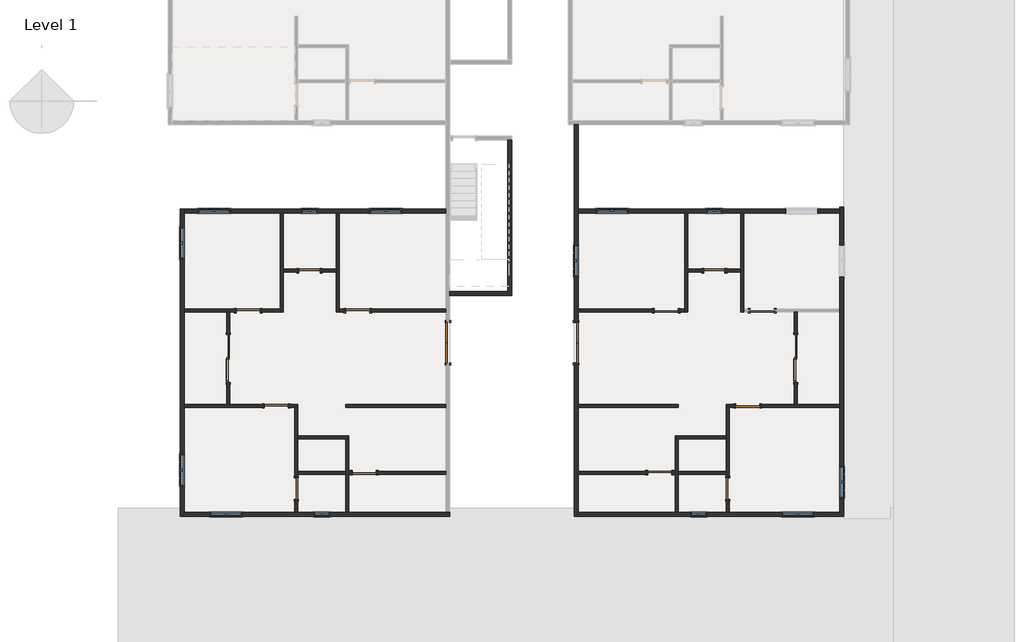
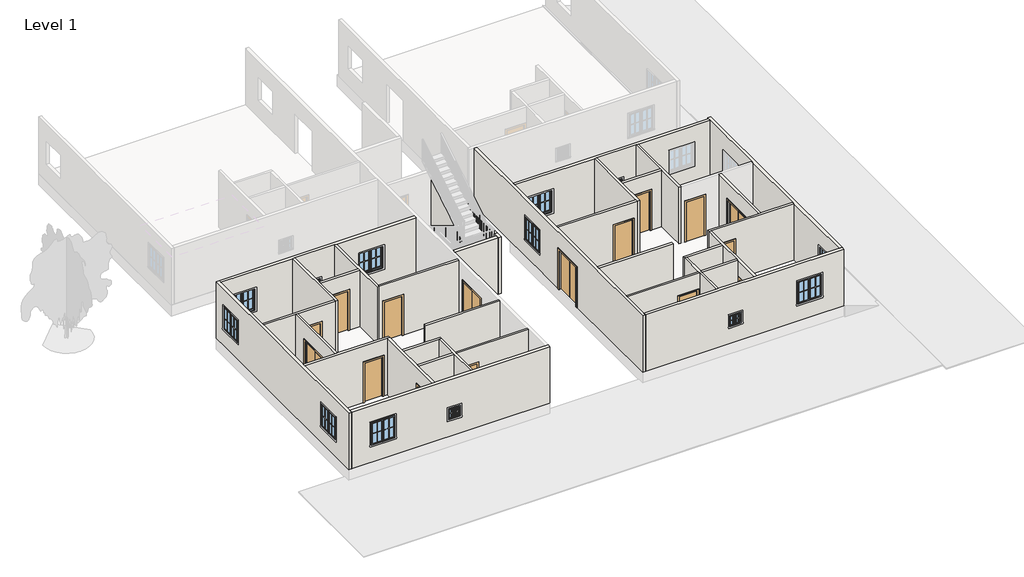
# One storey, part 1 of 7: 32 walls, 16 doors, 13 windows.
"""IFC4 building model written with IfcOpenShell, lengths in millimetres."""

from ifc_helpers import new_model, si_unit, frame, origin, origin_with_axes, place, context, project, spatial, polyline, outline, extrude, faceted_brep, transform, mapped, element, save
from components import door_a09c2f77, door_166d4031, door_d141acb4, door_e5f9f3c4, window_0c121b81, window_191d0cfb

model = new_model("IFC4")

# Units and contexts
model_context = context("Model", 3, world=origin())
ifc_project = project(units=[si_unit("LENGTHUNIT", "METRE", prefix="MILLI")], contexts=[model_context])

# Site, building, storey
site = spatial("IfcSite", under=ifc_project)
building = spatial("IfcBuilding", under=site)
storey = spatial("IfcBuildingStorey", under=building, Name="Level 1", Elevation=0.0)

# Doors
placement = place(None, origin())
door_shape = door_a09c2f77(model_context)
element("IfcDoor", 1, ObjectType="Door-Double-Flush_Panel : 60\" x 84\"", at=placement, inside=storey, context=model_context, shape_type="MappedRepresentation", body=[
    mapped(door_shape, transform((-3579.3844485, -6148.3564015, 0.0), x_axis=(0.0, 1.0, 0.0), y_axis=(-1.0, 0.0, 0.0), z_axis=(0.0, 0.0, 1.0))),
])
element("IfcDoor", 2, ObjectType="Door-Double-Flush_Panel : 60\" x 84\"", at=placement, inside=storey, context=model_context, shape_type="MappedRepresentation", body=[
    mapped(door_shape, transform((1297.4155515, -6148.3564015, 0.0), x_axis=(0.0, -1.0, 0.0), y_axis=(1.0, 0.0, 0.0), z_axis=(0.0, 0.0, 1.0))),
])
door_2_shape = door_166d4031(model_context)
element("IfcDoor", 3, ObjectType="Door-Double-Sliding : 72\" x 84\"", at=placement, inside=storey, context=model_context, shape_type="MappedRepresentation", body=[
    mapped(door_2_shape, transform((-11796.2844485, -6738.9064015, 0.0), x_axis=(0.0, 1.0, 0.0), y_axis=(-1.0, 0.0, 0.0), z_axis=(0.0, 0.0, 1.0))),
])
element("IfcDoor", 4, ObjectType="Door-Double-Sliding : 72\" x 84\"", at=placement, inside=storey, context=model_context, shape_type="MappedRepresentation", body=[
    mapped(door_2_shape, transform((9768.3155515, -6738.9064015, 0.0), x_axis=(0.0, 1.0, 0.0), y_axis=(-1.0, 0.0, 0.0), z_axis=(0.0, 0.0, 1.0))),
])
door_3_shape = door_d141acb4(model_context)
element("IfcDoor", 5, ObjectType="Single-Flush : 32\" x 84\"", at=placement, inside=storey, context=model_context, shape_type="MappedRepresentation", body=[
    mapped(door_3_shape, transform((-8829.5474256, -3405.1564015, 0.0), x_axis=(1.0, 0.0, 0.0), y_axis=(0.0, 1.0, 0.0), z_axis=(0.0, 0.0, 1.0))),
])
element("IfcDoor", 6, ObjectType="Single-Flush : 32\" x 84\"", at=placement, inside=storey, context=model_context, shape_type="MappedRepresentation", body=[
    mapped(door_3_shape, transform((-9338.8344485, -11698.2564015, 0.0), x_axis=(0.0, -1.0, 0.0), y_axis=(1.0, 0.0, 0.0), z_axis=(0.0, 0.0, 1.0))),
])
element("IfcDoor", 7, ObjectType="Single-Flush : 32\" x 84\"", at=placement, inside=storey, context=model_context, shape_type="MappedRepresentation", body=[
    mapped(door_3_shape, transform((7056.8655515, -11698.2564015, 0.0), x_axis=(0.0, 1.0, 0.0), y_axis=(-1.0, 0.0, 0.0), z_axis=(0.0, 0.0, 1.0))),
])
element("IfcDoor", 8, ObjectType="Single-Flush : 32\" x 84\"", at=placement, inside=storey, context=model_context, shape_type="MappedRepresentation", body=[
    mapped(door_3_shape, transform((6547.5785285, -3405.1564015, 0.0), x_axis=(1.0, 0.0, 0.0), y_axis=(0.0, 1.0, 0.0), z_axis=(0.0, 0.0, 1.0))),
])
door_4_shape = door_e5f9f3c4(model_context)
element("IfcDoor", 9, ObjectType="Single-Flush : 36\" x 84\"", at=placement, inside=storey, context=model_context, shape_type="MappedRepresentation", body=[
    mapped(door_4_shape, transform((-11161.2844485, -4929.1564015, 0.0), x_axis=(1.0, 0.0, 0.0), y_axis=(0.0, 1.0, 0.0), z_axis=(0.0, 0.0, 1.0))),
])
element("IfcDoor", 10, ObjectType="Single-Flush : 36\" x 84\"", at=placement, inside=storey, context=model_context, shape_type="MappedRepresentation", body=[
    mapped(door_4_shape, transform((-7007.0974256, -4929.1564015, 0.0), x_axis=(1.0, 0.0, 0.0), y_axis=(0.0, 1.0, 0.0), z_axis=(0.0, 0.0, 1.0))),
])
element("IfcDoor", 11, ObjectType="Single-Flush : 36\" x 84\"", at=placement, inside=storey, context=model_context, shape_type="MappedRepresentation", body=[
    mapped(door_4_shape, transform((-10100.8344485, -8548.6564015, 0.0), x_axis=(1.0, 0.0, 0.0), y_axis=(0.0, 1.0, 0.0), z_axis=(0.0, 0.0, 1.0))),
])
element("IfcDoor", 12, ObjectType="Single-Flush : 36\" x 84\"", at=placement, inside=storey, context=model_context, shape_type="MappedRepresentation", body=[
    mapped(door_4_shape, transform((-6748.0344485, -11088.6564015, 0.0), x_axis=(-1.0, 0.0, 0.0), y_axis=(0.0, -1.0, 0.0), z_axis=(0.0, 0.0, 1.0))),
])
element("IfcDoor", 13, ObjectType="Single-Flush : 36\" x 84\"", at=placement, inside=storey, context=model_context, shape_type="MappedRepresentation", body=[
    mapped(door_4_shape, transform((7818.8655515, -8548.6564015, 0.0), x_axis=(-1.0, 0.0, 0.0), y_axis=(0.0, -1.0, 0.0), z_axis=(0.0, 0.0, 1.0))),
])
element("IfcDoor", 14, ObjectType="Single-Flush : 36\" x 84\"", at=placement, inside=storey, context=model_context, shape_type="MappedRepresentation", body=[
    mapped(door_4_shape, transform((4466.0655515, -11088.6564015, 0.0), x_axis=(1.0, 0.0, 0.0), y_axis=(0.0, 1.0, 0.0), z_axis=(0.0, 0.0, 1.0))),
])
element("IfcDoor", 15, ObjectType="Single-Flush : 36\" x 84\"", at=placement, inside=storey, context=model_context, shape_type="MappedRepresentation", body=[
    mapped(door_4_shape, transform((4725.1285285, -4929.1564015, 0.0), x_axis=(-1.0, 0.0, 0.0), y_axis=(0.0, -1.0, 0.0), z_axis=(0.0, 0.0, 1.0))),
])
element("IfcDoor", 16, ObjectType="Single-Flush : 36\" x 84\"", at=placement, inside=storey, context=model_context, shape_type="MappedRepresentation", body=[
    mapped(door_4_shape, transform((8370.0285285, -4929.1564015, 0.0), x_axis=(-1.0, 0.0, 0.0), y_axis=(0.0, -1.0, 0.0), z_axis=(0.0, 0.0, 1.0))),
])

# Walls
element("IfcWall", 17, ObjectType="4.5\"", at=placement, inside=storey, context=model_context, shape_type="Brep", body=[
    faceted_brep([(-9947.1474256, -1214.4064015, 0.0), (-9947.1474256, -4872.0064015, 0.0), (-9947.1474256, -4986.3064015, 0.0), (-9947.1474256, -4986.3064015, 3048.0), (-9947.1474256, -4872.0064015, 3048.0), (-9947.1474256, -1214.4064015, 3048.0), (-9832.8474256, -1214.4064015, 0.0), (-9832.8474256, -1214.4064015, 3048.0), (-9832.8474256, -3348.0064015, 3048.0), (-9832.8474256, -3462.3064015, 3048.0), (-9832.8474256, -4986.3064015, 3048.0), (-9832.8474256, -4986.3064015, 0.0), (-9832.8474256, -3462.3064015, 0.0), (-9832.8474256, -3348.0064015, 0.0)], [[[0, 1, 2, 3, 4, 5]], [[6, 7, 8, 9, 10, 11, 12, 13]], [[2, 1, 0, 6, 13, 12, 11]], [[0, 5, 7, 6]], [[3, 2, 11, 10]], [[5, 4, 3, 10, 9, 8, 7]]]),
])
element("IfcWall", 18, ObjectType="4.5\"", at=placement, inside=storey, context=model_context, shape_type="Brep", body=[
    faceted_brep([(-9947.1474256, -4872.0064015, 0.0), (-10704.0844485, -4872.0064015, 0.0), (-10704.0844485, -4872.0064015, 2133.6), (-11618.4844485, -4872.0064015, 2133.6), (-11618.4844485, -4872.0064015, 0.0), (-13604.1663899, -4872.0064015, 0.0), (-13604.1663899, -4872.0064015, 3048.0), (-9947.1474256, -4872.0064015, 3048.0), (-10704.0844485, -4986.3064015, 2133.6), (-10704.0844485, -4986.3064015, 0.0), (-9947.1474256, -4986.3064015, 0.0), (-9947.1474256, -4986.3064015, 3048.0), (-11866.1344485, -4986.3064015, 3048.0), (-11980.4344485, -4986.3064015, 3048.0), (-13604.1663899, -4986.3064015, 3048.0), (-13604.1663899, -4986.3064015, 0.0), (-11980.4344485, -4986.3064015, 0.0), (-11866.1344485, -4986.3064015, 0.0), (-11618.4844485, -4986.3064015, 0.0), (-11618.4844485, -4986.3064015, 2133.6)], [[[0, 1, 2, 3, 4, 5, 6, 7]], [[8, 9, 10, 11, 12, 13, 14, 15, 16, 17, 18, 19]], [[10, 9, 1, 0]], [[18, 17, 16, 15, 5, 4]], [[0, 7, 11, 10]], [[6, 5, 15, 14]], [[2, 1, 9, 8]], [[3, 2, 8, 19]], [[4, 3, 19, 18]], [[7, 6, 14, 13, 12, 11]]]),
])
element("IfcWall", 19, ObjectType="4.5\"", at=placement, inside=storey, context=model_context, shape_type="SweptSolid", body=[
    extrude(outline(polyline([(-4986.3064015, 0.0), (-5824.5064015, 0.0), (-5824.5064015, 2133.6), (-7653.3064015, 2133.6), (-7653.3064015, 0.0), (-8491.5064015, 0.0), (-8491.5064015, 3048.0), (-4986.3064015, 3048.0), (-4986.3064015, 0.0)])), frame((-11980.4344485, 0.0, 0.0), z_axis=(1.0, 0.0, 0.0), x_axis=(0.0, 1.0, 0.0)), (0.0, 0.0, 1.0), 114.3),
])
element("IfcWall", 20, ObjectType="4.5\"", at=placement, inside=storey, context=model_context, shape_type="SweptSolid", body=[
    extrude(outline(polyline([(2133.6, -8423.1474256), (0.0, -8423.1474256), (0.0, -7826.2474256), (3048.0, -7826.2474256), (3048.0, -9832.8474256), (0.0, -9832.8474256), (0.0, -9235.9474256), (2133.6, -9235.9474256), (2133.6, -8423.1474256)])), frame((0.0, -3462.3064015, 0.0), z_axis=(0.0, 1.0, 0.0), x_axis=(0.0, 0.0, 1.0)), (0.0, 0.0, 1.0), 114.3),
])
element("IfcWall", 21, ObjectType="4.5\"", at=placement, inside=storey, context=model_context, shape_type="Brep", body=[
    faceted_brep([(-7826.2474256, -1214.4064015, 0.0), (-7826.2474256, -3348.0064015, 0.0), (-7826.2474256, -3462.3064015, 0.0), (-7826.2474256, -4986.3064015, 0.0), (-7826.2474256, -4986.3064015, 3048.0), (-7826.2474256, -3462.3064015, 3048.0), (-7826.2474256, -3348.0064015, 3048.0), (-7826.2474256, -1214.4064015, 3048.0), (-7711.9474256, -1214.4064015, 0.0), (-7711.9474256, -1214.4064015, 3048.0), (-7711.9474256, -4872.0064015, 3048.0), (-7711.9474256, -4986.3064015, 3048.0), (-7711.9474256, -4986.3064015, 0.0), (-7711.9474256, -4872.0064015, 0.0)], [[[0, 1, 2, 3, 4, 5, 6, 7]], [[8, 9, 10, 11, 12, 13]], [[3, 2, 1, 0, 8, 13, 12]], [[0, 7, 9, 8]], [[4, 3, 12, 11]], [[7, 6, 5, 4, 11, 10, 9]]]),
])
element("IfcWall", 22, ObjectType="4.5\"", at=placement, inside=storey, context=model_context, shape_type="SweptSolid", body=[
    extrude(outline(polyline([(2133.6, -6549.8974256), (0.0, -6549.8974256), (0.0, -3655.5844485), (3048.0, -3655.5844485), (3048.0, -7711.9474256), (0.0, -7711.9474256), (0.0, -7464.2974256), (2133.6, -7464.2974256), (2133.6, -6549.8974256)])), frame((0.0, -4986.3064015, 0.0), z_axis=(0.0, 1.0, 0.0), x_axis=(0.0, 0.0, 1.0)), (0.0, 0.0, 1.0), 114.3),
])
element("IfcWall", 23, ObjectType="4.5\"", at=placement, inside=storey, context=model_context, shape_type="Brep", body=[
    faceted_brep([(-9643.6344485, -8605.8064015, 2133.6), (-9643.6344485, -8605.8064015, 0.0), (-9395.9844485, -8605.8064015, 0.0), (-9281.6844485, -8605.8064015, 0.0), (-9281.6844485, -8605.8064015, 3048.0), (-9395.9844485, -8605.8064015, 3048.0), (-13604.1663899, -8605.8064015, 3048.0), (-13604.1663899, -8605.8064015, 0.0), (-10558.0344485, -8605.8064015, 0.0), (-10558.0344485, -8605.8064015, 2133.6), (-9281.6844485, -8491.5064015, 0.0), (-9643.6344485, -8491.5064015, 0.0), (-9643.6344485, -8491.5064015, 2133.6), (-10558.0344485, -8491.5064015, 2133.6), (-10558.0344485, -8491.5064015, 0.0), (-11866.1344485, -8491.5064015, 0.0), (-11980.4344485, -8491.5064015, 0.0), (-13604.1663899, -8491.5064015, 0.0), (-13604.1663899, -8491.5064015, 3048.0), (-11980.4344485, -8491.5064015, 3048.0), (-11866.1344485, -8491.5064015, 3048.0), (-9281.6844485, -8491.5064015, 3048.0)], [[[0, 1, 2, 3, 4, 5, 6, 7, 8, 9]], [[10, 11, 12, 13, 14, 15, 16, 17, 18, 19, 20, 21]], [[8, 7, 17, 16, 15, 14]], [[3, 2, 1, 11, 10]], [[7, 6, 18, 17]], [[4, 3, 10, 21]], [[12, 11, 1, 0]], [[13, 12, 0, 9]], [[14, 13, 9, 8]], [[6, 5, 4, 21, 20, 19, 18]]]),
])
element("IfcWall", 24, ObjectType="4.5\"", at=placement, inside=storey, context=model_context, shape_type="Brep", body=[
    faceted_brep([(-9395.9844485, -12104.6564015, 2133.6), (-9395.9844485, -12104.6564015, 0.0), (-9395.9844485, -12593.6064015, 0.0), (-9395.9844485, -12593.6064015, 3048.0), (-9395.9844485, -8605.8064015, 3048.0), (-9395.9844485, -8605.8064015, 0.0), (-9395.9844485, -11291.8564015, 0.0), (-9395.9844485, -11291.8564015, 2133.6), (-9281.6844485, -12593.6064015, 0.0), (-9281.6844485, -12104.6564015, 0.0), (-9281.6844485, -12104.6564015, 2133.6), (-9281.6844485, -11291.8564015, 2133.6), (-9281.6844485, -11291.8564015, 0.0), (-9281.6844485, -11145.8064015, 0.0), (-9281.6844485, -11031.5064015, 0.0), (-9281.6844485, -9812.3064015, 0.0), (-9281.6844485, -9698.0064015, 0.0), (-9281.6844485, -8605.8064015, 0.0), (-9281.6844485, -8605.8064015, 3048.0), (-9281.6844485, -9698.0064015, 3048.0), (-9281.6844485, -9812.3064015, 3048.0), (-9281.6844485, -11031.5064015, 3048.0), (-9281.6844485, -11145.8064015, 3048.0), (-9281.6844485, -12593.6064015, 3048.0)], [[[0, 1, 2, 3, 4, 5, 6, 7]], [[8, 9, 10, 11, 12, 13, 14, 15, 16, 17, 18, 19, 20, 21, 22, 23]], [[6, 5, 17, 16, 15, 14, 13, 12]], [[2, 1, 9, 8]], [[5, 4, 18, 17]], [[3, 2, 8, 23]], [[10, 9, 1, 0]], [[11, 10, 0, 7]], [[12, 11, 7, 6]], [[4, 3, 23, 22, 21, 20, 19, 18]]]),
])
element("IfcWall", 25, ObjectType="4.5\"", at=placement, inside=storey, context=model_context, shape_type="Brep", body=[
    faceted_brep([(-9281.6844485, -9812.3064015, 0.0), (-7452.8844485, -9812.3064015, 0.0), (-7338.5844485, -9812.3064015, 0.0), (-7338.5844485, -9812.3064015, 3048.0), (-7452.8844485, -9812.3064015, 3048.0), (-9281.6844485, -9812.3064015, 3048.0), (-9281.6844485, -9698.0064015, 0.0), (-9281.6844485, -9698.0064015, 3048.0), (-7338.5844485, -9698.0064015, 3048.0), (-7338.5844485, -9698.0064015, 0.0)], [[[0, 1, 2, 3, 4, 5]], [[6, 7, 8, 9]], [[2, 1, 0, 6, 9]], [[0, 5, 7, 6]], [[3, 2, 9, 8]], [[5, 4, 3, 8, 7]]]),
])
element("IfcWall", 26, ObjectType="4.5\"", at=placement, inside=storey, context=model_context, shape_type="Brep", body=[
    faceted_brep([(-7452.8844485, -9812.3064015, 0.0), (-7452.8844485, -11031.5064015, 0.0), (-7452.8844485, -11145.8064015, 0.0), (-7452.8844485, -12593.6064015, 0.0), (-7452.8844485, -12593.6064015, 3048.0), (-7452.8844485, -11145.8064015, 3048.0), (-7452.8844485, -11031.5064015, 3048.0), (-7452.8844485, -9812.3064015, 3048.0), (-7338.5844485, -9812.3064015, 0.0), (-7338.5844485, -9812.3064015, 3048.0), (-7338.5844485, -11031.5064015, 3048.0), (-7338.5844485, -11145.8064015, 3048.0), (-7338.5844485, -12593.6064015, 3048.0), (-7338.5844485, -12593.6064015, 0.0), (-7338.5844485, -11145.8064015, 0.0), (-7338.5844485, -11031.5064015, 0.0)], [[[0, 1, 2, 3, 4, 5, 6, 7]], [[8, 9, 10, 11, 12, 13, 14, 15]], [[3, 2, 1, 0, 8, 15, 14, 13]], [[0, 7, 9, 8]], [[4, 3, 13, 12]], [[7, 6, 5, 4, 12, 11, 10, 9]]]),
])
element("IfcWall", 27, ObjectType="4.5\"", at=placement, inside=storey, context=model_context, shape_type="SweptSolid", body=[
    extrude(outline(polyline([(0.0, -3655.5844485), (3048.0, -3655.5844485), (3048.0, -7338.5844485), (0.0, -7338.5844485), (0.0, -7205.2344485), (2133.6, -7205.2344485), (2133.6, -6290.8344485), (0.0, -6290.8344485), (0.0, -3655.5844485)])), frame((0.0, -11145.8064015, 0.0), z_axis=(0.0, 1.0, 0.0), x_axis=(0.0, 0.0, 1.0)), (0.0, 0.0, 1.0), 114.3),
    extrude(outline(polyline([(-9281.6844485, -11145.8064015), (-9281.6844485, -11031.5064015), (-7452.8844485, -11031.5064015), (-7452.8844485, -11145.8064015), (-9281.6844485, -11145.8064015)])), origin_with_axes(), (0.0, 0.0, 1.0), 3048.0),
])
element("IfcWall", 28, ObjectType="4.5\"", at=placement, inside=storey, context=model_context, shape_type="SweptSolid", body=[
    extrude(outline(polyline([(-3655.5844485, -8605.8064015), (-7452.8844485, -8605.8064015), (-7452.8844485, -8491.5064015), (-3655.5844485, -8491.5064015), (-3655.5844485, -8605.8064015)])), origin_with_axes(), (0.0, 0.0, 1.0), 3048.0),
])
element("IfcWall", 29, ObjectType="4.5\"", at=placement, inside=storey, context=model_context, shape_type="Brep", body=[
    faceted_brep([(5429.9785285, -1214.4064015, 0.0), (5429.9785285, -4872.0064015, 0.0), (5429.9785285, -4986.3064015, 0.0), (5429.9785285, -4986.3064015, 3048.0), (5429.9785285, -4872.0064015, 3048.0), (5429.9785285, -1214.4064015, 3048.0), (5544.2785285, -1214.4064015, 0.0), (5544.2785285, -1214.4064015, 3048.0), (5544.2785285, -3348.0064015, 3048.0), (5544.2785285, -3462.3064015, 3048.0), (5544.2785285, -4986.3064015, 3048.0), (5544.2785285, -4986.3064015, 0.0), (5544.2785285, -3462.3064015, 0.0), (5544.2785285, -3348.0064015, 0.0)], [[[0, 1, 2, 3, 4, 5]], [[6, 7, 8, 9, 10, 11, 12, 13]], [[2, 1, 0, 6, 13, 12, 11]], [[0, 5, 7, 6]], [[3, 2, 11, 10]], [[5, 4, 3, 10, 9, 8, 7]]]),
])
element("IfcWall", 30, ObjectType="4.5\"", at=placement, inside=storey, context=model_context, shape_type="SweptSolid", body=[
    extrude(outline(polyline([(0.0, 1373.6155515), (0.0, 4267.9285285), (2133.6, 4267.9285285), (2133.6, 5182.3285285), (0.0, 5182.3285285), (0.0, 5429.9785285), (3048.0, 5429.9785285), (3048.0, 1373.6155515), (0.0, 1373.6155515)])), frame((0.0, -4986.3064015, 0.0), z_axis=(0.0, 1.0, 0.0), x_axis=(0.0, 0.0, 1.0)), (0.0, 0.0, 1.0), 114.3),
])
element("IfcWall", 31, ObjectType="4.5\"", at=placement, inside=storey, context=model_context, shape_type="Brep", body=[
    faceted_brep([(7550.8785285, -1214.4064015, 0.0), (7550.8785285, -3348.0064015, 0.0), (7550.8785285, -3462.3064015, 0.0), (7550.8785285, -4986.3064015, 0.0), (7550.8785285, -4986.3064015, 3048.0), (7550.8785285, -3462.3064015, 3048.0), (7550.8785285, -3348.0064015, 3048.0), (7550.8785285, -1214.4064015, 3048.0), (7665.1785285, -1214.4064015, 0.0), (7665.1785285, -1214.4064015, 3048.0), (7665.1785285, -4872.0064015, 3048.0), (7665.1785285, -4986.3064015, 3048.0), (7665.1785285, -4986.3064015, 0.0), (7665.1785285, -4872.0064015, 0.0)], [[[0, 1, 2, 3, 4, 5, 6, 7]], [[8, 9, 10, 11, 12, 13]], [[3, 2, 1, 0, 8, 13, 12]], [[0, 7, 9, 8]], [[4, 3, 12, 11]], [[7, 6, 5, 4, 11, 10, 9]]]),
])
element("IfcWall", 32, ObjectType="4.5\"", at=placement, inside=storey, context=model_context, shape_type="SweptSolid", body=[
    extrude(outline(polyline([(2133.6, 6953.9785285), (0.0, 6953.9785285), (0.0, 7550.8785285), (3048.0, 7550.8785285), (3048.0, 5544.2785285), (0.0, 5544.2785285), (0.0, 6141.1785285), (2133.6, 6141.1785285), (2133.6, 6953.9785285)])), frame((0.0, -3462.3064015, 0.0), z_axis=(0.0, 1.0, 0.0), x_axis=(0.0, 0.0, 1.0)), (0.0, 0.0, 1.0), 114.3),
])
element("IfcWall", 33, ObjectType="4.5\"", at=placement, inside=storey, context=model_context, shape_type="SweptSolid", body=[
    extrude(outline(polyline([(-4986.3064015, 0.0), (-5824.5064015, 0.0), (-5824.5064015, 2133.6), (-7653.3064015, 2133.6), (-7653.3064015, 0.0), (-8491.5064015, 0.0), (-8491.5064015, 3048.0), (-4986.3064015, 3048.0), (-4986.3064015, 0.0)])), frame((9584.1655515, 0.0, 0.0), z_axis=(1.0, 0.0, 0.0), x_axis=(0.0, 1.0, 0.0)), (0.0, 0.0, 1.0), 114.3),
])
element("IfcWall", 34, ObjectType="4.5\"", at=placement, inside=storey, context=model_context, shape_type="Brep", body=[
    faceted_brep([(7361.6655515, -8491.5064015, 2133.6), (7361.6655515, -8491.5064015, 0.0), (6999.7155515, -8491.5064015, 0.0), (6999.7155515, -8491.5064015, 3048.0), (9584.1655515, -8491.5064015, 3048.0), (9698.4655515, -8491.5064015, 3048.0), (11322.7785285, -8491.5064015, 3048.0), (11322.7785285, -8491.5064015, 0.0), (9698.4655515, -8491.5064015, 0.0), (9584.1655515, -8491.5064015, 0.0), (8276.0655515, -8491.5064015, 0.0), (8276.0655515, -8491.5064015, 2133.6), (6999.7155515, -8605.8064015, 0.0), (7114.0155515, -8605.8064015, 0.0), (7361.6655515, -8605.8064015, 0.0), (7361.6655515, -8605.8064015, 2133.6), (8276.0655515, -8605.8064015, 2133.6), (8276.0655515, -8605.8064015, 0.0), (11322.7785285, -8605.8064015, 0.0), (11322.7785285, -8605.8064015, 3048.0), (7114.0155515, -8605.8064015, 3048.0), (6999.7155515, -8605.8064015, 3048.0)], [[[0, 1, 2, 3, 4, 5, 6, 7, 8, 9, 10, 11]], [[12, 13, 14, 15, 16, 17, 18, 19, 20, 21]], [[2, 1, 14, 13, 12]], [[10, 9, 8, 7, 18, 17]], [[7, 6, 19, 18]], [[3, 2, 12, 21]], [[15, 14, 1, 0]], [[16, 15, 0, 11]], [[17, 16, 11, 10]], [[6, 5, 4, 3, 21, 20, 19]]]),
])
element("IfcWall", 35, ObjectType="4.5\"", at=placement, inside=storey, context=model_context, shape_type="Brep", body=[
    faceted_brep([(6999.7155515, -8605.8064015, 0.0), (6999.7155515, -9698.0064015, 0.0), (6999.7155515, -9812.3064015, 0.0), (6999.7155515, -11031.5064015, 0.0), (6999.7155515, -11145.8064015, 0.0), (6999.7155515, -11291.8564015, 0.0), (6999.7155515, -11291.8564015, 2133.6), (6999.7155515, -12104.6564015, 2133.6), (6999.7155515, -12104.6564015, 0.0), (6999.7155515, -12593.6064015, 0.0), (6999.7155515, -12593.6064015, 3048.0), (6999.7155515, -11145.8064015, 3048.0), (6999.7155515, -11031.5064015, 3048.0), (6999.7155515, -9812.3064015, 3048.0), (6999.7155515, -9698.0064015, 3048.0), (6999.7155515, -8605.8064015, 3048.0), (7114.0155515, -11291.8564015, 2133.6), (7114.0155515, -11291.8564015, 0.0), (7114.0155515, -8605.8064015, 0.0), (7114.0155515, -8605.8064015, 3048.0), (7114.0155515, -12593.6064015, 3048.0), (7114.0155515, -12593.6064015, 0.0), (7114.0155515, -12104.6564015, 0.0), (7114.0155515, -12104.6564015, 2133.6)], [[[0, 1, 2, 3, 4, 5, 6, 7, 8, 9, 10, 11, 12, 13, 14, 15]], [[16, 17, 18, 19, 20, 21, 22, 23]], [[22, 21, 9, 8]], [[18, 17, 5, 4, 3, 2, 1, 0]], [[0, 15, 19, 18]], [[10, 9, 21, 20]], [[6, 5, 17, 16]], [[7, 6, 16, 23]], [[8, 7, 23, 22]], [[15, 14, 13, 12, 11, 10, 20, 19]]]),
])
element("IfcWall", 36, ObjectType="4.5\"", at=placement, inside=storey, context=model_context, shape_type="Brep", body=[
    faceted_brep([(6999.7155515, -9698.0064015, 0.0), (5056.6155515, -9698.0064015, 0.0), (5056.6155515, -9698.0064015, 3048.0), (6999.7155515, -9698.0064015, 3048.0), (6999.7155515, -9812.3064015, 0.0), (6999.7155515, -9812.3064015, 3048.0), (5170.9155515, -9812.3064015, 3048.0), (5056.6155515, -9812.3064015, 3048.0), (5056.6155515, -9812.3064015, 0.0), (5170.9155515, -9812.3064015, 0.0)], [[[0, 1, 2, 3]], [[4, 5, 6, 7, 8, 9]], [[1, 0, 4, 9, 8]], [[0, 3, 5, 4]], [[2, 1, 8, 7]], [[3, 2, 7, 6, 5]]]),
])
element("IfcWall", 37, ObjectType="4.5\"", at=placement, inside=storey, context=model_context, shape_type="Brep", body=[
    faceted_brep([(5056.6155515, -9812.3064015, 0.0), (5056.6155515, -11031.5064015, 0.0), (5056.6155515, -11145.8064015, 0.0), (5056.6155515, -12593.6064015, 0.0), (5056.6155515, -12593.6064015, 3048.0), (5056.6155515, -11145.8064015, 3048.0), (5056.6155515, -11031.5064015, 3048.0), (5056.6155515, -9812.3064015, 3048.0), (5170.9155515, -9812.3064015, 0.0), (5170.9155515, -9812.3064015, 3048.0), (5170.9155515, -11031.5064015, 3048.0), (5170.9155515, -11145.8064015, 3048.0), (5170.9155515, -12593.6064015, 3048.0), (5170.9155515, -12593.6064015, 0.0), (5170.9155515, -11145.8064015, 0.0), (5170.9155515, -11031.5064015, 0.0)], [[[0, 1, 2, 3, 4, 5, 6, 7]], [[8, 9, 10, 11, 12, 13, 14, 15]], [[3, 2, 1, 0, 8, 15, 14, 13]], [[0, 7, 9, 8]], [[4, 3, 13, 12]], [[7, 6, 5, 4, 12, 11, 10, 9]]]),
])
element("IfcWall", 38, ObjectType="4.5\"", at=placement, inside=storey, context=model_context, shape_type="SweptSolid", body=[
    extrude(outline(polyline([(3048.0, 1373.6155515), (0.0, 1373.6155515), (0.0, 4008.8655515), (2133.6, 4008.8655515), (2133.6, 4923.2655515), (0.0, 4923.2655515), (0.0, 5056.6155515), (3048.0, 5056.6155515), (3048.0, 1373.6155515)])), frame((0.0, -11145.8064015, 0.0), z_axis=(0.0, 1.0, 0.0), x_axis=(0.0, 0.0, 1.0)), (0.0, 0.0, 1.0), 114.3),
    extrude(outline(polyline([(6999.7155515, -11031.5064015), (6999.7155515, -11145.8064015), (5170.9155515, -11145.8064015), (5170.9155515, -11031.5064015), (6999.7155515, -11031.5064015)])), origin_with_axes(), (0.0, 0.0, 1.0), 3048.0),
])
element("IfcWall", 39, ObjectType="4.5\"", at=placement, inside=storey, context=model_context, shape_type="SweptSolid", body=[
    extrude(outline(polyline([(5170.9155515, -8605.8064015), (1373.6155515, -8605.8064015), (1373.6155515, -8491.5064015), (5170.9155515, -8491.5064015), (5170.9155515, -8605.8064015)])), origin_with_axes(), (0.0, 0.0, 1.0), 3048.0),
])
element("IfcWall", 40, ObjectType="6\"", at=placement, inside=storey, context=model_context, shape_type="Brep", body=[
    faceted_brep([(-13756.5663899, -1055.4730729, 0.0), (-13756.5663899, -12746.0064015, 0.0), (-13756.5663899, -12746.0064015, 3048.0), (-13756.5663899, -1055.4730729, 3048.0), (-13756.5663899, -1747.8317701, 2133.6), (-13756.5663899, -2967.0317701, 2133.6), (-13756.5663899, -2967.0317701, 914.4), (-13756.5663899, -1747.8317701, 914.4), (-13756.5663899, -10383.8317701, 2133.6), (-13756.5663899, -11603.0317701, 2133.6), (-13756.5663899, -11603.0317701, 914.4), (-13756.5663899, -10383.8317701, 914.4), (-13604.1663899, -1055.4730729, 0.0), (-13604.1663899, -1055.4730729, 3048.0), (-13604.1663899, -1062.0064015, 3048.0), (-13604.1663899, -1214.4064015, 3048.0), (-13604.1663899, -4872.0064015, 3048.0), (-13604.1663899, -4986.3064015, 3048.0), (-13604.1663899, -8491.5064015, 3048.0), (-13604.1663899, -8605.8064015, 3048.0), (-13604.1663899, -12593.6064015, 3048.0), (-13604.1663899, -12746.0064015, 3048.0), (-13604.1663899, -12746.0064015, 0.0), (-13604.1663899, -12593.6064015, 0.0), (-13604.1663899, -8605.8064015, 0.0), (-13604.1663899, -8491.5064015, 0.0), (-13604.1663899, -4986.3064015, 0.0), (-13604.1663899, -4872.0064015, 0.0), (-13604.1663899, -1214.4064015, 0.0), (-13604.1663899, -1062.0064015, 0.0), (-13604.1663899, -1747.8317701, 2133.6), (-13604.1663899, -1747.8317701, 914.4), (-13604.1663899, -2967.0317701, 914.4), (-13604.1663899, -2967.0317701, 2133.6), (-13604.1663899, -10383.8317701, 2133.6), (-13604.1663899, -10383.8317701, 914.4), (-13604.1663899, -11603.0317701, 914.4), (-13604.1663899, -11603.0317701, 2133.6)], [[[0, 1, 2, 3], [4, 5, 6, 7], [8, 9, 10, 11]], [[12, 13, 14, 15, 16, 17, 18, 19, 20, 21, 22, 23, 24, 25, 26, 27, 28, 29], [30, 31, 32, 33], [34, 35, 36, 37]], [[1, 0, 12, 29, 28, 27, 26, 25, 24, 23, 22]], [[0, 3, 13, 12]], [[2, 1, 22, 21]], [[31, 30, 4, 7]], [[32, 31, 7, 6]], [[33, 32, 6, 5]], [[30, 33, 5, 4]], [[35, 34, 8, 11]], [[36, 35, 11, 10]], [[37, 36, 10, 9]], [[34, 37, 9, 8]], [[3, 2, 21, 20, 19, 18, 17, 16, 15, 14, 13]]]),
])
element("IfcWall", 41, ObjectType="6\"", at=placement, inside=storey, context=model_context, shape_type="Brep", body=[
    faceted_brep([(-13604.1663899, -12746.0064015, 0.0), (-3503.1844485, -12746.0064015, 0.0), (-3503.1844485, -12746.0064015, 3048.0), (-13604.1663899, -12746.0064015, 3048.0), (-12614.1474256, -12746.0064015, 2133.6), (-11394.9474256, -12746.0064015, 2133.6), (-11394.9474256, -12746.0064015, 914.4), (-12614.1474256, -12746.0064015, 914.4), (-8672.0844485, -12746.0064015, 1524.0), (-8062.4844485, -12746.0064015, 1524.0), (-8062.4844485, -12746.0064015, 914.4), (-8672.0844485, -12746.0064015, 914.4), (-13604.1663899, -12593.6064015, 0.0), (-13604.1663899, -12593.6064015, 3048.0), (-9395.9844485, -12593.6064015, 3048.0), (-9281.6844485, -12593.6064015, 3048.0), (-7452.8844485, -12593.6064015, 3048.0), (-7338.5844485, -12593.6064015, 3048.0), (-3655.5844485, -12593.6064015, 3048.0), (-3503.1844485, -12593.6064015, 3048.0), (-3503.1844485, -12593.6064015, 0.0), (-3655.5844485, -12593.6064015, 0.0), (-7338.5844485, -12593.6064015, 0.0), (-7452.8844485, -12593.6064015, 0.0), (-9281.6844485, -12593.6064015, 0.0), (-9395.9844485, -12593.6064015, 0.0), (-12614.1474256, -12593.6064015, 2133.6), (-12614.1474256, -12593.6064015, 914.4), (-11394.9474256, -12593.6064015, 914.4), (-11394.9474256, -12593.6064015, 2133.6), (-8672.0844485, -12593.6064015, 1524.0), (-8672.0844485, -12593.6064015, 914.4), (-8062.4844485, -12593.6064015, 914.4), (-8062.4844485, -12593.6064015, 1524.0)], [[[0, 1, 2, 3], [4, 5, 6, 7], [8, 9, 10, 11]], [[12, 13, 14, 15, 16, 17, 18, 19, 20, 21, 22, 23, 24, 25], [26, 27, 28, 29], [30, 31, 32, 33]], [[1, 0, 12, 25, 24, 23, 22, 21, 20]], [[0, 3, 13, 12]], [[2, 1, 20, 19]], [[27, 26, 4, 7]], [[28, 27, 7, 6]], [[29, 28, 6, 5]], [[26, 29, 5, 4]], [[31, 30, 8, 11]], [[32, 31, 11, 10]], [[33, 32, 10, 9]], [[30, 33, 9, 8]], [[3, 2, 19, 18, 17, 16, 15, 14, 13]]]),
])
element("IfcWall", 42, ObjectType="6\"", at=placement, inside=storey, context=model_context, shape_type="Brep", body=[
    faceted_brep([(-13604.1663899, -1214.4064015, 0.0), (-9947.1474256, -1214.4064015, 0.0), (-9832.8474256, -1214.4064015, 0.0), (-7826.2474256, -1214.4064015, 0.0), (-7711.9474256, -1214.4064015, 0.0), (-3655.5844485, -1214.4064015, 0.0), (-3655.5844485, -1214.4064015, 3048.0), (-7711.9474256, -1214.4064015, 3048.0), (-7826.2474256, -1214.4064015, 3048.0), (-9832.8474256, -1214.4064015, 3048.0), (-9947.1474256, -1214.4064015, 3048.0), (-13604.1663899, -1214.4064015, 3048.0), (-5330.6974256, -1214.4064015, 2133.6), (-5330.6974256, -1214.4064015, 914.4), (-6549.8974256, -1214.4064015, 914.4), (-6549.8974256, -1214.4064015, 2133.6), (-8524.7474256, -1214.4064015, 1524.0), (-8524.7474256, -1214.4064015, 914.4), (-9134.3474256, -1214.4064015, 914.4), (-9134.3474256, -1214.4064015, 1524.0), (-11852.1474256, -1214.4064015, 2133.6), (-11852.1474256, -1214.4064015, 914.4), (-13071.3474256, -1214.4064015, 914.4), (-13071.3474256, -1214.4064015, 2133.6), (-3655.5844485, -1062.0064015, 0.0), (-13604.1663899, -1062.0064015, 0.0), (-13604.1663899, -1062.0064015, 3048.0), (-3655.5844485, -1062.0064015, 3048.0), (-5330.6974256, -1062.0064015, 2133.6), (-6549.8974256, -1062.0064015, 2133.6), (-6549.8974256, -1062.0064015, 914.4), (-5330.6974256, -1062.0064015, 914.4), (-8524.7474256, -1062.0064015, 1524.0), (-9134.3474256, -1062.0064015, 1524.0), (-9134.3474256, -1062.0064015, 914.4), (-8524.7474256, -1062.0064015, 914.4), (-11852.1474256, -1062.0064015, 914.4), (-11852.1474256, -1062.0064015, 2133.6), (-13071.3474256, -1062.0064015, 2133.6), (-13071.3474256, -1062.0064015, 914.4)], [[[0, 1, 2, 3, 4, 5, 6, 7, 8, 9, 10, 11], [12, 13, 14, 15], [16, 17, 18, 19], [20, 21, 22, 23]], [[24, 25, 26, 27], [28, 29, 30, 31], [32, 33, 34, 35], [36, 37, 38, 39]], [[5, 4, 3, 2, 1, 0, 25, 24]], [[6, 5, 24, 27]], [[13, 12, 28, 31]], [[14, 13, 31, 30]], [[15, 14, 30, 29]], [[12, 15, 29, 28]], [[17, 16, 32, 35]], [[18, 17, 35, 34]], [[19, 18, 34, 33]], [[16, 19, 33, 32]], [[11, 10, 9, 8, 7, 6, 27, 26]], [[20, 37, 36, 21]], [[21, 36, 39, 22]], [[37, 20, 23, 38]], [[38, 23, 22, 39]], [[0, 11, 26, 25]]]),
])
element("IfcWall", 43, ObjectType="6\"", at=placement, inside=storey, context=model_context, shape_type="Brep", body=[
    faceted_brep([(1221.2155515, 2138.3935985, 3048.0), (1221.2155515, 2138.3935985, 0.0), (1221.2155515, -5386.3564015, 0.0), (1221.2155515, -5386.3564015, 2133.6), (1221.2155515, -6910.3564015, 2133.6), (1221.2155515, -6910.3564015, 0.0), (1221.2155515, -12746.0064015, 0.0), (1221.2155515, -12746.0064015, 3048.0), (1221.2155515, -2424.0814015, 2133.6), (1221.2155515, -3643.2814015, 2133.6), (1221.2155515, -3643.2814015, 914.4), (1221.2155515, -2424.0814015, 914.4), (1373.6155515, 2138.3935985, 0.0), (1373.6155515, 2138.3935985, 3048.0), (1373.6155515, -1062.0064015, 3048.0), (1373.6155515, -1214.4064015, 3048.0), (1373.6155515, -4872.0064015, 3048.0), (1373.6155515, -4986.3064015, 3048.0), (1373.6155515, -8491.5064015, 3048.0), (1373.6155515, -8605.8064015, 3048.0), (1373.6155515, -11031.5064015, 3048.0), (1373.6155515, -11145.8064015, 3048.0), (1373.6155515, -12593.6064015, 3048.0), (1373.6155515, -12746.0064015, 3048.0), (1373.6155515, -12746.0064015, 0.0), (1373.6155515, -12593.6064015, 0.0), (1373.6155515, -11145.8064015, 0.0), (1373.6155515, -11031.5064015, 0.0), (1373.6155515, -8605.8064015, 0.0), (1373.6155515, -8491.5064015, 0.0), (1373.6155515, -6910.3564015, 0.0), (1373.6155515, -6910.3564015, 2133.6), (1373.6155515, -5386.3564015, 2133.6), (1373.6155515, -5386.3564015, 0.0), (1373.6155515, -4986.3064015, 0.0), (1373.6155515, -4872.0064015, 0.0), (1373.6155515, -1214.4064015, 0.0), (1373.6155515, -1062.0064015, 0.0), (1373.6155515, -2424.0814015, 2133.6), (1373.6155515, -2424.0814015, 914.4), (1373.6155515, -3643.2814015, 914.4), (1373.6155515, -3643.2814015, 2133.6)], [[[0, 1, 2, 3, 4, 5, 6, 7], [8, 9, 10, 11]], [[12, 13, 14, 15, 16, 17, 18, 19, 20, 21, 22, 23, 24, 25, 26, 27, 28, 29, 30, 31, 32, 33, 34, 35, 36, 37], [38, 39, 40, 41]], [[1, 12, 37, 36, 35, 34, 33, 2]], [[24, 6, 5, 30, 29, 28, 27, 26, 25]], [[1, 0, 13, 12]], [[7, 6, 24, 23]], [[39, 38, 8, 11]], [[40, 39, 11, 10]], [[41, 40, 10, 9]], [[38, 41, 9, 8]], [[4, 31, 30, 5]], [[31, 4, 3, 32]], [[32, 3, 2, 33]], [[0, 7, 23, 22, 21, 20, 19, 18, 17, 16, 15, 14, 13]]]),
])
element("IfcWall", 44, ObjectType="6\"", at=placement, inside=storey, context=model_context, shape_type="Brep", body=[
    faceted_brep([(1373.6155515, -12746.0064015, 0.0), (11475.1785285, -12746.0064015, 0.0), (11475.1785285, -12746.0064015, 3048.0), (1373.6155515, -12746.0064015, 3048.0), (9112.9785285, -12746.0064015, 2133.6), (10332.1785285, -12746.0064015, 2133.6), (10332.1785285, -12746.0064015, 914.4), (9112.9785285, -12746.0064015, 914.4), (5647.1655515, -12746.0064015, 1524.0), (6256.7655515, -12746.0064015, 1524.0), (6256.7655515, -12746.0064015, 914.4), (5647.1655515, -12746.0064015, 914.4), (1373.6155515, -12593.6064015, 0.0), (1373.6155515, -12593.6064015, 3048.0), (5056.6155515, -12593.6064015, 3048.0), (5170.9155515, -12593.6064015, 3048.0), (6999.7155515, -12593.6064015, 3048.0), (7114.0155515, -12593.6064015, 3048.0), (11322.7785285, -12593.6064015, 3048.0), (11475.1785285, -12593.6064015, 3048.0), (11475.1785285, -12593.6064015, 0.0), (11322.7785285, -12593.6064015, 0.0), (7114.0155515, -12593.6064015, 0.0), (6999.7155515, -12593.6064015, 0.0), (5170.9155515, -12593.6064015, 0.0), (5056.6155515, -12593.6064015, 0.0), (9112.9785285, -12593.6064015, 2133.6), (9112.9785285, -12593.6064015, 914.4), (10332.1785285, -12593.6064015, 914.4), (10332.1785285, -12593.6064015, 2133.6), (5647.1655515, -12593.6064015, 1524.0), (5647.1655515, -12593.6064015, 914.4), (6256.7655515, -12593.6064015, 914.4), (6256.7655515, -12593.6064015, 1524.0)], [[[0, 1, 2, 3], [4, 5, 6, 7], [8, 9, 10, 11]], [[12, 13, 14, 15, 16, 17, 18, 19, 20, 21, 22, 23, 24, 25], [26, 27, 28, 29], [30, 31, 32, 33]], [[1, 0, 12, 25, 24, 23, 22, 21, 20]], [[0, 3, 13, 12]], [[2, 1, 20, 19]], [[27, 26, 4, 7]], [[28, 27, 7, 6]], [[29, 28, 6, 5]], [[26, 29, 5, 4]], [[31, 30, 8, 11]], [[32, 31, 11, 10]], [[33, 32, 10, 9]], [[30, 33, 9, 8]], [[3, 2, 19, 18, 17, 16, 15, 14, 13]]]),
])
element("IfcWall", 45, ObjectType="6\"", at=placement, inside=storey, context=model_context, shape_type="Brep", body=[
    faceted_brep([(11475.1785285, -12593.6064015, 0.0), (11475.1785285, -985.8064015, 0.0), (11475.1785285, -985.8064015, 3048.0), (11475.1785285, -12593.6064015, 3048.0), (11475.1785285, -3643.2814015, 2133.6), (11475.1785285, -2424.0814015, 2133.6), (11475.1785285, -2424.0814015, 914.4), (11475.1785285, -3643.2814015, 914.4), (11475.1785285, -12060.2064015, 2133.6), (11475.1785285, -10841.0064015, 2133.6), (11475.1785285, -10841.0064015, 914.4), (11475.1785285, -12060.2064015, 914.4), (11322.7785285, -12593.6064015, 0.0), (11322.7785285, -12593.6064015, 3048.0), (11322.7785285, -8605.8064015, 3048.0), (11322.7785285, -8491.5064015, 3048.0), (11322.7785285, -4986.3064015, 3048.0), (11322.7785285, -4872.0064015, 3048.0), (11322.7785285, -1214.4064015, 3048.0), (11322.7785285, -1062.0064015, 3048.0), (11322.7785285, -985.8064015, 3048.0), (11322.7785285, -985.8064015, 0.0), (11322.7785285, -1062.0064015, 0.0), (11322.7785285, -1214.4064015, 0.0), (11322.7785285, -4872.0064015, 0.0), (11322.7785285, -4986.3064015, 0.0), (11322.7785285, -8491.5064015, 0.0), (11322.7785285, -8605.8064015, 0.0), (11322.7785285, -3643.2814015, 2133.6), (11322.7785285, -3643.2814015, 914.4), (11322.7785285, -2424.0814015, 914.4), (11322.7785285, -2424.0814015, 2133.6), (11322.7785285, -12060.2064015, 2133.6), (11322.7785285, -12060.2064015, 914.4), (11322.7785285, -10841.0064015, 914.4), (11322.7785285, -10841.0064015, 2133.6)], [[[0, 1, 2, 3], [4, 5, 6, 7], [8, 9, 10, 11]], [[12, 13, 14, 15, 16, 17, 18, 19, 20, 21, 22, 23, 24, 25, 26, 27], [28, 29, 30, 31], [32, 33, 34, 35]], [[1, 0, 12, 27, 26, 25, 24, 23, 22, 21]], [[2, 1, 21, 20]], [[0, 3, 13, 12]], [[29, 28, 4, 7]], [[30, 29, 7, 6]], [[31, 30, 6, 5]], [[28, 31, 5, 4]], [[33, 32, 8, 11]], [[34, 33, 11, 10]], [[35, 34, 10, 9]], [[32, 35, 9, 8]], [[3, 2, 20, 19, 18, 17, 16, 15, 14, 13]]]),
])
element("IfcWall", 46, ObjectType="6\"", at=placement, inside=storey, context=model_context, shape_type="Brep", body=[
    faceted_brep([(11322.7785285, -1062.0064015, 0.0), (1373.6155515, -1062.0064015, 0.0), (1373.6155515, -1062.0064015, 3048.0), (11322.7785285, -1062.0064015, 3048.0), (3278.6155515, -1062.0064015, 2133.6), (2059.4155515, -1062.0064015, 2133.6), (2059.4155515, -1062.0064015, 914.4), (3278.6155515, -1062.0064015, 914.4), (10484.5785285, -1062.0064015, 2133.6), (9265.3785285, -1062.0064015, 2133.6), (9265.3785285, -1062.0064015, 914.4), (10484.5785285, -1062.0064015, 914.4), (6852.3785285, -1062.0064015, 1524.0), (6242.7785285, -1062.0064015, 1524.0), (6242.7785285, -1062.0064015, 914.4), (6852.3785285, -1062.0064015, 914.4), (11322.7785285, -1214.4064015, 0.0), (11322.7785285, -1214.4064015, 3048.0), (7665.1785285, -1214.4064015, 3048.0), (7550.8785285, -1214.4064015, 3048.0), (5544.2785285, -1214.4064015, 3048.0), (5429.9785285, -1214.4064015, 3048.0), (1373.6155515, -1214.4064015, 3048.0), (1373.6155515, -1214.4064015, 0.0), (5429.9785285, -1214.4064015, 0.0), (5544.2785285, -1214.4064015, 0.0), (7550.8785285, -1214.4064015, 0.0), (7665.1785285, -1214.4064015, 0.0), (3278.6155515, -1214.4064015, 2133.6), (3278.6155515, -1214.4064015, 914.4), (2059.4155515, -1214.4064015, 914.4), (2059.4155515, -1214.4064015, 2133.6), (10484.5785285, -1214.4064015, 2133.6), (10484.5785285, -1214.4064015, 914.4), (9265.3785285, -1214.4064015, 914.4), (9265.3785285, -1214.4064015, 2133.6), (6852.3785285, -1214.4064015, 1524.0), (6852.3785285, -1214.4064015, 914.4), (6242.7785285, -1214.4064015, 914.4), (6242.7785285, -1214.4064015, 1524.0)], [[[0, 1, 2, 3], [4, 5, 6, 7], [8, 9, 10, 11], [12, 13, 14, 15]], [[16, 17, 18, 19, 20, 21, 22, 23, 24, 25, 26, 27], [28, 29, 30, 31], [32, 33, 34, 35], [36, 37, 38, 39]], [[1, 0, 16, 27, 26, 25, 24, 23]], [[2, 1, 23, 22]], [[0, 3, 17, 16]], [[29, 28, 4, 7]], [[30, 29, 7, 6]], [[31, 30, 6, 5]], [[28, 31, 5, 4]], [[33, 32, 8, 11]], [[34, 33, 11, 10]], [[35, 34, 10, 9]], [[32, 35, 9, 8]], [[37, 36, 12, 15]], [[38, 37, 15, 14]], [[39, 38, 14, 13]], [[36, 39, 13, 12]], [[3, 2, 22, 21, 20, 19, 18, 17]]]),
])
element("IfcWall", 47, ObjectType="6\"", at=placement, inside=storey, context=model_context, shape_type="Brep", body=[
    faceted_brep([(-1293.3844485, 1560.7269271, 0.0), (-1293.3844485, -4205.0730729, 0.0), (-1293.3844485, -4357.4730729, 0.0), (-1293.3844485, -4357.4730729, 3048.0), (-1293.3844485, -4205.0730729, 3048.0), (-1293.3844485, -4001.8730729, 3048.0), (-1293.3844485, 1560.7269271, 3048.0), (-1140.9844485, 1560.7269271, 0.0), (-1140.9844485, 1560.7269271, 3048.0), (-1140.9844485, -4001.8730729, 3048.0), (-1140.9844485, -4357.4730729, 3048.0), (-1140.9844485, -4357.4730729, 0.0)], [[[0, 1, 2, 3, 4, 5, 6]], [[7, 8, 9, 10, 11]], [[2, 1, 0, 7, 11]], [[0, 6, 8, 7]], [[3, 2, 11, 10]], [[6, 5, 9, 8]], [[5, 4, 3, 10, 9]]]),
])
element("IfcWall", 48, ObjectType="6\"", at=placement, inside=storey, context=model_context, shape_type="SweptSolid", body=[
    extrude(outline(polyline([(-3503.1844485, -4205.0730729), (-1293.3844485, -4205.0730729), (-1293.3844485, -4357.4730729), (-3503.1844485, -4357.4730729), (-3503.1844485, -4205.0730729)])), origin_with_axes(), (0.0, 0.0, 1.0), 3048.0),
])

# Windows
window_shape = window_0c121b81(model_context)
element("IfcWindow", 49, ObjectType="Window-Casement-Double : 24\" x 24\"", at=placement, inside=storey, context=model_context, shape_type="MappedRepresentation", body=[
    mapped(window_shape, transform((-8829.5474256, -1138.2064015, 0.0), x_axis=(1.0, 0.0, 0.0), y_axis=(0.0, 1.0, 0.0), z_axis=(0.0, 0.0, 1.0))),
])
element("IfcWindow", 50, ObjectType="Window-Casement-Double : 24\" x 24\"", at=placement, inside=storey, context=model_context, shape_type="MappedRepresentation", body=[
    mapped(window_shape, transform((-8367.2844485, -12669.8064015, 0.0), x_axis=(-1.0, 0.0, 0.0), y_axis=(0.0, -1.0, 0.0), z_axis=(0.0, 0.0, 1.0))),
])
element("IfcWindow", 51, ObjectType="Window-Casement-Double : 24\" x 24\"", at=placement, inside=storey, context=model_context, shape_type="MappedRepresentation", body=[
    mapped(window_shape, transform((5951.9655515, -12669.8064015, 0.0), x_axis=(-1.0, 0.0, 0.0), y_axis=(0.0, -1.0, 0.0), z_axis=(0.0, 0.0, 1.0))),
])
element("IfcWindow", 52, ObjectType="Window-Casement-Double : 24\" x 24\"", at=placement, inside=storey, context=model_context, shape_type="MappedRepresentation", body=[
    mapped(window_shape, transform((6547.5785285, -1138.2064015, 0.0), x_axis=(1.0, 0.0, 0.0), y_axis=(0.0, 1.0, 0.0), z_axis=(0.0, 0.0, 1.0))),
])
window_2_shape = window_191d0cfb(model_context)
element("IfcWindow", 53, ObjectType="Window-Casement-Double : 48\" x 48\"", at=placement, inside=storey, context=model_context, shape_type="MappedRepresentation", body=[
    mapped(window_2_shape, transform((-12461.7474256, -1138.2064015, 0.0), x_axis=(1.0, 0.0, 0.0), y_axis=(0.0, 1.0, 0.0), z_axis=(0.0, 0.0, 1.0))),
])
element("IfcWindow", 54, ObjectType="Window-Casement-Double : 48\" x 48\"", at=placement, inside=storey, context=model_context, shape_type="MappedRepresentation", body=[
    mapped(window_2_shape, transform((-13680.3663899, -2357.4317701, 0.0), x_axis=(0.0, 1.0, 0.0), y_axis=(-1.0, 0.0, 0.0), z_axis=(0.0, 0.0, 1.0))),
])
element("IfcWindow", 55, ObjectType="Window-Casement-Double : 48\" x 48\"", at=placement, inside=storey, context=model_context, shape_type="MappedRepresentation", body=[
    mapped(window_2_shape, transform((-5940.2974256, -1138.2064015, 0.0), x_axis=(1.0, 0.0, 0.0), y_axis=(0.0, 1.0, 0.0), z_axis=(0.0, 0.0, 1.0))),
])
element("IfcWindow", 56, ObjectType="Window-Casement-Double : 48\" x 48\"", at=placement, inside=storey, context=model_context, shape_type="MappedRepresentation", body=[
    mapped(window_2_shape, transform((-13680.3663899, -10993.4317701, 0.0), x_axis=(0.0, 1.0, 0.0), y_axis=(-1.0, 0.0, 0.0), z_axis=(0.0, 0.0, 1.0))),
])
element("IfcWindow", 57, ObjectType="Window-Casement-Double : 48\" x 48\"", at=placement, inside=storey, context=model_context, shape_type="MappedRepresentation", body=[
    mapped(window_2_shape, transform((-12004.5474256, -12669.8064015, 0.0), x_axis=(-1.0, 0.0, 0.0), y_axis=(0.0, -1.0, 0.0), z_axis=(0.0, 0.0, 1.0))),
])
element("IfcWindow", 58, ObjectType="Window-Casement-Double : 48\" x 48\"", at=placement, inside=storey, context=model_context, shape_type="MappedRepresentation", body=[
    mapped(window_2_shape, transform((2669.0155515, -1138.2064015, 0.0), x_axis=(1.0, 0.0, 0.0), y_axis=(0.0, 1.0, 0.0), z_axis=(0.0, 0.0, 1.0))),
])
element("IfcWindow", 59, ObjectType="Window-Casement-Double : 48\" x 48\"", at=placement, inside=storey, context=model_context, shape_type="MappedRepresentation", body=[
    mapped(window_2_shape, transform((1297.4155515, -3033.6814015, 0.0), x_axis=(0.0, 1.0, 0.0), y_axis=(-1.0, 0.0, 0.0), z_axis=(0.0, 0.0, 1.0))),
])
element("IfcWindow", 60, ObjectType="Window-Casement-Double : 48\" x 48\"", at=placement, inside=storey, context=model_context, shape_type="MappedRepresentation", body=[
    mapped(window_2_shape, transform((11398.9785285, -11450.6064015, 0.0), x_axis=(0.0, -1.0, 0.0), y_axis=(1.0, 0.0, 0.0), z_axis=(0.0, 0.0, 1.0))),
])
element("IfcWindow", 61, ObjectType="Window-Casement-Double : 48\" x 48\"", at=placement, inside=storey, context=model_context, shape_type="MappedRepresentation", body=[
    mapped(window_2_shape, transform((9722.5785285, -12669.8064015, 0.0), x_axis=(-1.0, 0.0, 0.0), y_axis=(0.0, -1.0, 0.0), z_axis=(0.0, 0.0, 1.0))),
])

save(model, "model.ifc")

# Revit data of these elements
# Type "Door-Double-Flush_Panel : 60\" x 84\""
#   Type Mark = "9"
#   Construction Type Id = "DOOR"
#   Assembly Code = "C1020"
#   Analytic Construction = "Wooden"
#   Thickness = 0' - 2"
#   Thermal Resistance (R) = 2.5876 (h·ft²·°F)/BTU
#   Swing Angle [instance default] = 90.00°
#   Panel Width = 2' - 6"
#   Heat Transfer Coefficient (U) = 0.3865 BTU/(h·ft²·°F)
#   Height = 7' - 0"
#   Trim Projection Ext = 0' - 1"
#   Trim Projection Int = 0' - 1"
#   Trim Width = 0' - 3"
#   Width = 5' - 0"
#   Define Thermal Properties by = 1
#   Panel Material = Wood - Birch - Solid Stained Light Low Gloss
#   Trim Material = Paint - Sienna
#   Visual Light Transmittance = 0
#   Solar Heat Gain Coefficient = 0
#   Function = (empty or 0)
#   Wall Closure = (empty or 0)
# Type "Door-Double-Sliding : 72\" x 84\""
#   Type Mark = "8"
#   Construction Type Id = "opn-d45"
#   Assembly Code = "C1020"
#   Analytic Construction = "Wood frame, double glass door "
#   Thickness = 0' - 2"
#   Thermal Resistance (R) = 1.8150 (h·ft²·°F)/BTU
#   Heat Transfer Coefficient (U) = 0.5510 BTU/(h·ft²·°F)
#   Height = 7' - 0"
#   Rail Width = 0' - 2"
#   Stiles = 0' - 2"
#   Trim Projection Ext = 0' - 1"
#   Trim Projection Int = 0' - 1"
#   Trim Width = 0' - 3"
#   Width = 6' - 0"
#   Define Thermal Properties by = 1
#   Glazing = Glass
#   Panel Material = Wood - Birch - Solid Stained Light Low Gloss
#   Trim Material = Paint - Sienna
#   Visual Light Transmittance = 0
#   Solar Heat Gain Coefficient = 0
#   Function = (empty or 0)
#   Wall Closure = (empty or 0)
# Type "Single-Flush : 32\" x 84\""
#   Type Mark = "3"
#   Construction Type Id = "MDOOR"
#   Assembly Code = "C1020"
#   Analytic Construction = "Metal"
#   Thickness = 0' - 2"
#   Heat Transfer Coefficient (U) = 0.651978 BTU/(h·ft²·°F)
#   Height = 7' - 0"
#   Trim Projection Ext = 0' - 1"
#   Trim Projection Int = 0' - 1"
#   Trim Width = 0' - 3"
#   Width = 2' - 8"
#   Define Thermal Properties by = 1
#   Define Thermal Properties by = 1
#   Door Material = Door - Panel
#   Frame Material = Door - Frame
#   Visual Light Transmittance = 0
#   Solar Heat Gain Coefficient = 0
#   Function = (empty or 0)
#   Wall Closure = (empty or 0)
# Type "Single-Flush : 36\" x 84\""
#   Type Mark = "1"
#   Construction Type Id = "MDOOR"
#   Assembly Code = "C1020"
#   Analytic Construction = "Metal"
#   Thickness = 0' - 2"
#   Heat Transfer Coefficient (U) = 0.651978 BTU/(h·ft²·°F)
#   Height = 7' - 0"
#   Trim Projection Ext = 0' - 1"
#   Trim Projection Int = 0' - 1"
#   Trim Width = 0' - 3"
#   Width = 3' - 0"
#   Define Thermal Properties by = 1
#   Define Thermal Properties by = 1
#   Door Material = Door - Panel
#   Frame Material = Door - Frame
#   Visual Light Transmittance = 0
#   Solar Heat Gain Coefficient = 0
#   Function = (empty or 0)
#   Wall Closure = (empty or 0)
# Type "4.5\""
#   Assembly Code = "B2010"
#   Layers, outside or top first: 0' - 4 1/2" "4.5\" WALL" (function 1)
# Type "6\""
#   Assembly Code = "B2010"
#   Layers, outside or top first: 0' - 6" "6\" WALL" (function 1)
# Type "Window-Casement-Double : 24\" x 24\""
#   Type Mark = "14"
#   Fire Rating = "0.5h"
#   Assembly Code = "B2020100"
#   Analytic Construction = "Double glazing - domestic"
#   Frame Extension [instance default] = 0' - 0 1/4"
#   Window Inset [instance default] = 0' - 0"
#   Wall Thickness [instance default] = 0' - 6"
#   Interior Wall Closure [instance default] = 0' - 2 1/4"
#   Half Width = 1' - 0"
#   Visual Light Transmittance = 0.81
#   Thermal Resistance (R) = 1.8146 (h·ft²·°F)/BTU
#   Solar Heat Gain Coefficient = 0.76
#   Rough Width = 2' - 0 1/2"
#   Rough Height = 2' - 0 1/2"
#   Height = 2' - 0"
#   Heat Transfer Coefficient (U) = 0.5511 BTU/(h·ft²·°F)
#   Exterior Wall Closure [instance default] = 0' - 1 1/4"
#   Extension Jamb [instance default] = 0' - 2 1/4"
#   Default Sill Height = 3' - 0"
#   Width = 2' - 0"
#   Define Thermal Properties by = 0
#   Muntin Visibility = yes
#   Interior Trim Visibility [instance default] = yes
#   Exterior Trim Visibility [instance default] = yes
#   Extension Jamb Visibility [instance default] = yes
#   Interior Trim Material = Wood - Stained
#   Muntin Pattern = Muntin Pattern_2x2 : Muntin Pattern_2x2
#   Interior Trim = Trim-Window-Interior-Flat : Picture Frame
#   Interior Frame Material = Wood - Stained
#   Glass Panel Material = Glass
#   Exterior Trim Material = Clad - White
#   Exterior Trim = Trim-Window-Exterior-Flat : with Sill
#   Exterior Frame Material = Clad - White
#   Wall Closure = (empty or 0)
# Type "Window-Casement-Double : 48\" x 48\""
#   Type Mark = "16"
#   Fire Rating = "0.5h"
#   Assembly Code = "B2020100"
#   Analytic Construction = "Double glazing - domestic"
#   Frame Extension [instance default] = 0' - 0 1/4"
#   Window Inset [instance default] = 0' - 0"
#   Wall Thickness [instance default] = 0' - 6"
#   Interior Wall Closure [instance default] = 0' - 2 1/4"
#   Half Width = 2' - 0"
#   Visual Light Transmittance = 0.81
#   Thermal Resistance (R) = 1.8146 (h·ft²·°F)/BTU
#   Solar Heat Gain Coefficient = 0.76
#   Rough Width = 4' - 0 1/2"
#   Rough Height = 4' - 0 1/2"
#   Height = 4' - 0"
#   Heat Transfer Coefficient (U) = 0.5511 BTU/(h·ft²·°F)
#   Exterior Wall Closure [instance default] = 0' - 1 1/4"
#   Extension Jamb [instance default] = 0' - 2 1/4"
#   Default Sill Height = 3' - 0"
#   Width = 4' - 0"
#   Define Thermal Properties by = 0
#   Muntin Visibility = yes
#   Interior Trim Visibility [instance default] = yes
#   Exterior Trim Visibility [instance default] = yes
#   Extension Jamb Visibility [instance default] = yes
#   Interior Trim Material = Wood - Stained
#   Muntin Pattern = Muntin Pattern_2x2 : Muntin Pattern_2x2
#   Interior Trim = Trim-Window-Interior-Flat : Picture Frame
#   Interior Frame Material = Wood - Stained
#   Glass Panel Material = Glass
#   Exterior Trim Material = Clad - White
#   Exterior Trim = Trim-Window-Exterior-Flat : with Sill
#   Exterior Frame Material = Clad - White
#   Wall Closure = (empty or 0)
# Elements 1, 2 (IfcDoor, "Door-Double-Flush_Panel : 60\" x 84\"")
#   Swing Angle = 90.00°
#   Phase Created = New Construction
#   Materials on its faces: "Paint - Sienna", "Wood - Birch - Solid Stained Light Low Gloss"
# Elements 3, 4 (IfcDoor, "Door-Double-Sliding : 72\" x 84\"")
#   Phase Created = New Construction
#   Materials on its faces: "Paint - Sienna", "Wood - Birch - Solid Stained Light Low Gloss", "Glass"
# Elements 5, 6, 7, 8 (IfcDoor, "Single-Flush : 32\" x 84\"")
#   Phase Created = New Construction
#   Materials on its faces: "Door - Frame", "Door - Panel"
# Elements 9, 10, 11, 12, 13, 14, 15, 16 (IfcDoor, "Single-Flush : 36\" x 84\"")
#   Phase Created = New Construction
#   Materials on its faces: "Door - Frame", "Door - Panel"
# Elements 17, 18, 19, 20, 21, 22, 23, 24, 25, 26, 27, 28, 29, 30, 31, 32, 33, 34, 35, 36, 37, 38, 39 (IfcWall, "4.5\"")
#   Top Offset = 0' - 0"
#   Base Offset = 0' - 0"
#   Unconnected Height = 10' - 0"
#   wall height = 10' - 0"
#   Phase Created = New Construction
#   Base Constraint = Level 1
#   Materials on its faces: "4.5\" WALL"
# Elements 40, 41, 42, 43, 44, 45, 46, 47, 48 (IfcWall, "6\"")
#   Top Offset = 0' - 0"
#   Base Offset = 0' - 0"
#   Unconnected Height = 10' - 0"
#   wall height = 10' - 0"
#   Phase Created = New Construction
#   Base Constraint = Level 1
#   Materials on its faces: "6\" WALL"
# Element 49 (IfcWindow, "Window-Casement-Double : 24\" x 24\"")
#   Mark = "26"
#   Window Inset = 0' - 0"
#   Interior Wall Closure = 0' - 2 1/4"
#   Frame Extension = 0' - 0 1/4"
#   Exterior Wall Closure = 0' - 1 1/4"
#   Interior Trim Visibility = yes
#   Exterior Trim Visibility = yes
#   Phase Created = New Construction
#   Materials on its faces: "Wood - Stained", "Glass", "Clad - White"
# Element 50 (IfcWindow, "Window-Casement-Double : 24\" x 24\"")
#   Mark = "27"
#   Window Inset = 0' - 0"
#   Interior Wall Closure = 0' - 2 1/4"
#   Frame Extension = 0' - 0 1/4"
#   Exterior Wall Closure = 0' - 1 1/4"
#   Interior Trim Visibility = yes
#   Exterior Trim Visibility = yes
#   Phase Created = New Construction
#   Materials on its faces: "Wood - Stained", "Glass", "Clad - White"
# Element 51 (IfcWindow, "Window-Casement-Double : 24\" x 24\"")
#   Mark = "28"
#   Window Inset = 0' - 0"
#   Interior Wall Closure = 0' - 2 1/4"
#   Frame Extension = 0' - 0 1/4"
#   Exterior Wall Closure = 0' - 1 1/4"
#   Interior Trim Visibility = yes
#   Exterior Trim Visibility = yes
#   Phase Created = New Construction
#   Materials on its faces: "Wood - Stained", "Glass", "Clad - White"
# Element 52 (IfcWindow, "Window-Casement-Double : 24\" x 24\"")
#   Mark = "29"
#   Window Inset = 0' - 0"
#   Interior Wall Closure = 0' - 2 1/4"
#   Frame Extension = 0' - 0 1/4"
#   Exterior Wall Closure = 0' - 1 1/4"
#   Interior Trim Visibility = yes
#   Exterior Trim Visibility = yes
#   Phase Created = New Construction
#   Materials on its faces: "Wood - Stained", "Glass", "Clad - White"
# Element 53 (IfcWindow, "Window-Casement-Double : 48\" x 48\"")
#   Mark = "12"
#   Window Inset = 0' - 0"
